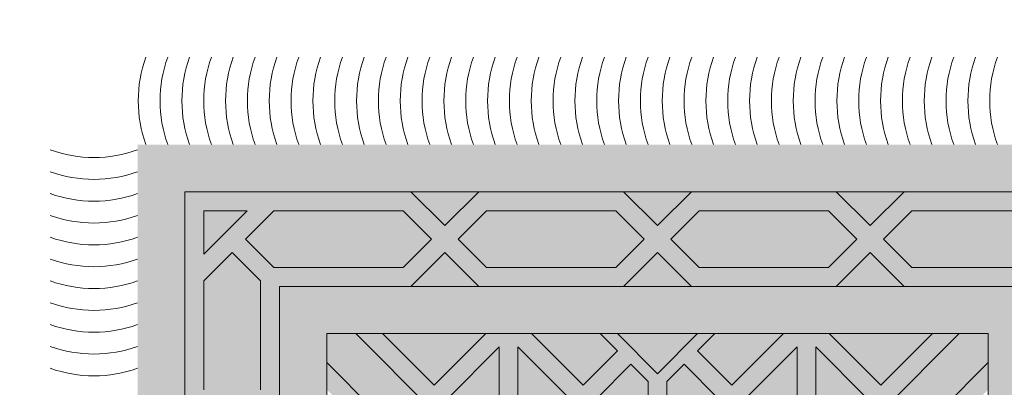
# Model space of a CAD drawing. Units: inches. Extents: x 844 to 2234, y 346 to 1084.
# Tile 21 of 93: x 1114.25 to 1127.54, y 705.06 to 710.02. Entities that reach past the tile are written whole.
import ezdxf

# ---------------------------------------------------------------- set-up
doc = ezdxf.new("R2010")
doc.units = ezdxf.units.IN
doc.header["$MEASUREMENT"] = 0
for name, color, linetype, lineweight in [('A-ANNO-DIMS', 2, 'Continuous', 18), ('furniture', 8, 'Continuous', 18), ('RA-AP-01$0$INT', 35, 'Continuous', 5)]:
    doc.layers.add(name, color=color, linetype=linetype, lineweight=lineweight)
doc.layers.add('RA-AP-01$0$FURN', color=3, linetype='Continuous')
doc.styles.get("Standard").update_dxf_attribs({"font": 'arial.ttf'})
doc.dimstyles.get("Standard").update_dxf_attribs({"dimtxt": 6, "dimasz": 3, "dimexe": 0.18, "dimexo": 0.0625, "dimgap": 0.09, "dimtad": 0, "dimtih": 1, "dimtoh": 1, "dimdec": 1, "dimzin": 0, "dimdsep": 46, "dimlunit": 3, "dimtxsty": 'Standard', "dimblk": 'ARCHTICK', "dimcen": 0.09, "dimadec": 0, "dimazin": 0, "dimtfac": 1, "dimtdec": 1, "dimtofl": 0, "dimtmove": 0, "dimatfit": 3, "dimfxl": 1, "dimtolj": 1, "dimtzin": 0, "dimarcsym": 0})

# ---------------------------------------------------------------- blocks, each defined once
blk = doc.blocks.new('A$C18D01794')
at = {"layer": 'RA-AP-01$0$INT'}
h = blk.add_hatch(color=256, dxfattribs=at)
h.paths.add_polyline_path([(4.3552, -6.1567), (4.3552, -8.0567), (5.4552, -8.0567), (5.4552, -6.1567)])
h.paths.add_polyline_path([(4.4052, -8.0067), (4.4052, -6.2067), (5.4052, -6.2067), (5.4052, -8.0067)], flags=16)
h = blk.add_hatch(color=256, dxfattribs=at)
h.paths.add_polyline_path([(4.5052, -7.5855), (4.4693, -7.5496), (4.5052, -7.5138), (4.5052, -7.382), (4.4693, -7.3461), (4.5052, -7.3102), (4.5052, -7.1784), (4.4693, -7.1426), (4.5052, -7.1067), (4.4769, -7.1067), (4.4552, -7.1284), (4.4335, -7.1067), (4.4052, -7.1067), (4.4411, -7.1426), (4.4052, -7.1784), (4.4052, -7.3102), (4.4411, -7.3461), (4.4052, -7.382), (4.4052, -7.5138), (4.4411, -7.5496), (4.4052, -7.5855), (4.4052, -7.7173), (4.4411, -7.7532), (4.4052, -7.789), (4.4052, -8.0067), (4.6443, -8.0067), (4.6802, -7.9709), (4.7161, -8.0067), (4.8693, -8.0067), (4.9052, -7.9709), (4.9411, -8.0067), (5.0943, -8.0067), (5.1302, -7.9709), (5.1661, -8.0067), (5.4052, -8.0067), (5.4052, -7.789), (5.3693, -7.7532), (5.4052, -7.7173), (5.4052, -7.5855), (5.3693, -7.5496), (5.4052, -7.5138), (5.4052, -7.382), (5.3693, -7.3461), (5.4052, -7.3102), (5.4052, -7.1784), (5.3693, -7.1426), (5.4052, -7.1067), (5.3769, -7.1067), (5.3552, -7.1284), (5.3335, -7.1067), (5.3052, -7.1067), (5.3411, -7.1426), (5.3052, -7.1784), (5.3052, -7.3102), (5.3411, -7.3461), (5.3052, -7.382), (5.3052, -7.5138), (5.3411, -7.5496), (5.3052, -7.5855), (5.3052, -7.7173), (5.3411, -7.7532), (5.3052, -7.789), (5.3052, -7.9067), (5.1661, -7.9067), (5.1302, -7.9426), (5.0943, -7.9067), (4.9411, -7.9067), (4.9052, -7.9426), (4.8693, -7.9067), (4.7161, -7.9067), (4.6802, -7.9426), (4.6443, -7.9067), (4.5052, -7.9067), (4.5052, -7.789), (4.4693, -7.7532), (4.5052, -7.7173)])
h.paths.add_polyline_path([(4.4852, -7.709), (4.4552, -7.739), (4.4252, -7.709), (4.4252, -7.5938), (4.4552, -7.5638), (4.4852, -7.5938)], flags=16)
h.paths.add_polyline_path([(4.4552, -7.7673), (4.4852, -7.7973), (4.4852, -7.9126), (4.4552, -7.9426), (4.4252, -7.9126), (4.4252, -7.7973)], flags=16)
h.paths.add_polyline_path([(4.4552, -7.5355), (4.4252, -7.5055), (4.4252, -7.3902), (4.4552, -7.3602), (4.4852, -7.3902), (4.4852, -7.5055)], flags=16)
h.paths.add_polyline_path([(4.4993, -7.9267), (4.6361, -7.9267), (4.6661, -7.9567), (4.6361, -7.9867), (4.4993, -7.9867), (4.4693, -7.9567)], flags=16)
h.paths.add_polyline_path([(4.4252, -7.9409), (4.4711, -7.9867), (4.4252, -7.9867)], flags=16)
h.paths.add_polyline_path([(4.4552, -7.332), (4.4252, -7.302), (4.4252, -7.1867), (4.4552, -7.1567), (4.4852, -7.1867), (4.4852, -7.302)], flags=16)
h.paths.add_polyline_path([(4.7243, -7.9267), (4.8611, -7.9267), (4.8911, -7.9567), (4.8611, -7.9867), (4.7243, -7.9867), (4.6943, -7.9567)], flags=16)
h.paths.add_polyline_path([(4.9193, -7.9567), (4.9493, -7.9267), (5.0861, -7.9267), (5.1161, -7.9567), (5.0861, -7.9867), (4.9493, -7.9867)], flags=16)
h.paths.add_polyline_path([(5.1443, -7.9567), (5.1743, -7.9267), (5.3111, -7.9267), (5.3411, -7.9567), (5.3111, -7.9867), (5.1743, -7.9867)], flags=16)
h.paths.add_polyline_path([(5.3252, -7.5938), (5.3552, -7.5638), (5.3852, -7.5938), (5.3852, -7.709), (5.3552, -7.739), (5.3252, -7.709)], flags=16)
h.paths.add_polyline_path([(5.3252, -7.7973), (5.3552, -7.7673), (5.3852, -7.7973), (5.3852, -7.9126), (5.3552, -7.9426), (5.3252, -7.9126)], flags=16)
h.paths.add_polyline_path([(5.3252, -7.5055), (5.3252, -7.3902), (5.3552, -7.3602), (5.3852, -7.3902), (5.3852, -7.5055), (5.3552, -7.5355)], flags=16)
h.paths.add_polyline_path([(5.3252, -7.302), (5.3252, -7.1867), (5.3552, -7.1567), (5.3852, -7.1867), (5.3852, -7.302), (5.3552, -7.332)], flags=16)
h.paths.add_polyline_path([(5.3393, -7.9867), (5.3852, -7.9409), (5.3852, -7.9867)], flags=16)
h = blk.add_hatch(color=256, dxfattribs=at)
h.paths.add_polyline_path([(4.4693, -7.1426), (4.5052, -7.1784), (4.5052, -7.1067)])
h.paths.add_polyline_path([(4.4552, -7.1284), (4.4769, -7.1067), (4.4335, -7.1067)])
h.paths.add_polyline_path([(4.4052, -7.1784), (4.4411, -7.1426), (4.4052, -7.1067)])
h.paths.add_polyline_path([(4.4252, -7.302), (4.4552, -7.332), (4.4852, -7.302), (4.4852, -7.1867), (4.4552, -7.1567), (4.4252, -7.1867)])
h.paths.add_polyline_path([(4.5052, -7.382), (4.5052, -7.3102), (4.4693, -7.3461)])
h.paths.add_polyline_path([(4.4252, -7.5055), (4.4552, -7.5355), (4.4852, -7.5055), (4.4852, -7.3902), (4.4552, -7.3602), (4.4252, -7.3902)])
h.paths.add_polyline_path([(4.4252, -7.709), (4.4552, -7.739), (4.4852, -7.709), (4.4852, -7.5938), (4.4552, -7.5638), (4.4252, -7.5938)])
h.paths.add_polyline_path([(4.4693, -7.5496), (4.5052, -7.5855), (4.5052, -7.5138)])
h.paths.add_polyline_path([(4.4052, -7.5855), (4.4411, -7.5496), (4.4052, -7.5138)])
h.paths.add_polyline_path([(4.4052, -7.789), (4.4411, -7.7532), (4.4052, -7.7173)])
h.paths.add_polyline_path([(4.4693, -7.7532), (4.5052, -7.789), (4.5052, -7.7173)])
h.paths.add_polyline_path([(4.4252, -7.9126), (4.4552, -7.9426), (4.4852, -7.9126), (4.4852, -7.7973), (4.4552, -7.7673), (4.4252, -7.7973)])
h.paths.add_polyline_path([(4.4252, -7.9867), (4.4711, -7.9867), (4.4252, -7.9409)])
h.paths.add_polyline_path([(4.4993, -7.9867), (4.6361, -7.9867), (4.6661, -7.9567), (4.6361, -7.9267), (4.4993, -7.9267), (4.4693, -7.9567)])
h.paths.add_polyline_path([(4.6802, -7.9426), (4.7161, -7.9067), (4.6443, -7.9067)])
h.paths.add_polyline_path([(4.6443, -8.0067), (4.7161, -8.0067), (4.6802, -7.9709)])
h.paths.add_polyline_path([(4.7243, -7.9867), (4.8611, -7.9867), (4.8911, -7.9567), (4.8611, -7.9267), (4.7243, -7.9267), (4.6943, -7.9567)])
h.paths.add_polyline_path([(4.9052, -7.9426), (4.9411, -7.9067), (4.8693, -7.9067)])
h.paths.add_polyline_path([(4.8693, -8.0067), (4.9411, -8.0067), (4.9052, -7.9709)])
h.paths.add_polyline_path([(4.9493, -7.9867), (5.0861, -7.9867), (5.1161, -7.9567), (5.0861, -7.9267), (4.9493, -7.9267), (4.9193, -7.9567)])
h.paths.add_polyline_path([(5.1302, -7.9426), (5.1661, -7.9067), (5.0943, -7.9067)])
h.paths.add_polyline_path([(5.0943, -8.0067), (5.1661, -8.0067), (5.1302, -7.9709)])
h.paths.add_polyline_path([(5.1743, -7.9867), (5.3111, -7.9867), (5.3411, -7.9567), (5.3111, -7.9267), (5.1743, -7.9267), (5.1443, -7.9567)])
h.paths.add_polyline_path([(5.3252, -7.9126), (5.3552, -7.9426), (5.3852, -7.9126), (5.3852, -7.7973), (5.3552, -7.7673), (5.3252, -7.7973)])
h.paths.add_polyline_path([(5.3393, -7.9867), (5.3852, -7.9867), (5.3852, -7.9409)])
h.paths.add_polyline_path([(5.3252, -7.709), (5.3552, -7.739), (5.3852, -7.709), (5.3852, -7.5938), (5.3552, -7.5638), (5.3252, -7.5938)])
h.paths.add_polyline_path([(5.3052, -7.789), (5.3411, -7.7532), (5.3052, -7.7173)])
h.paths.add_polyline_path([(5.3693, -7.7532), (5.4052, -7.789), (5.4052, -7.7173)])
h.paths.add_polyline_path([(5.4052, -7.5855), (5.4052, -7.5138), (5.3693, -7.5496)])
h.paths.add_polyline_path([(5.3052, -7.5855), (5.3411, -7.5496), (5.3052, -7.5138)])
h.paths.add_polyline_path([(5.3252, -7.5055), (5.3552, -7.5355), (5.3852, -7.5055), (5.3852, -7.3902), (5.3552, -7.3602), (5.3252, -7.3902)])
h.paths.add_polyline_path([(5.3052, -7.382), (5.3411, -7.3461), (5.3052, -7.3102)])
h.paths.add_polyline_path([(5.3252, -7.302), (5.3552, -7.332), (5.3852, -7.302), (5.3852, -7.1867), (5.3552, -7.1567), (5.3252, -7.1867)])
h.paths.add_polyline_path([(5.4046, -7.3813, -0.001218), (5.4052, -7.3811), (5.4052, -7.3102), (5.3693, -7.3461)])
h.paths.add_polyline_path([(5.3693, -7.1426), (5.4052, -7.1784), (5.4052, -7.1067)])
h.paths.add_polyline_path([(5.3552, -7.1284), (5.3769, -7.1067), (5.3335, -7.1067)])
h.paths.add_polyline_path([(5.3052, -7.1784), (5.3411, -7.1426), (5.3052, -7.1067)])
blk.add_hatch(color=256, dxfattribs=at).paths.add_polyline_path([(4.5052, -7.9067), (5.3052, -7.9067), (5.3052, -7.1067), (5.2552, -7.1067), (5.2552, -7.8567), (4.5552, -7.8567), (4.5552, -7.1067), (4.5052, -7.1067)])
h = blk.add_hatch(color=256, dxfattribs=at)
h.paths.add_polyline_path([(4.5859, -7.8567), (4.6142, -7.8567), (4.6688, -7.8021), (4.7235, -7.8567), (4.7718, -7.8567), (4.8264, -7.8021), (4.8628, -7.8384), (4.8445, -7.8567), (4.8628, -7.8567), (4.9052, -7.8143), (4.9476, -7.8567), (4.9659, -7.8567), (4.9476, -7.8384), (4.984, -7.8021), (5.0386, -7.8567), (5.0869, -7.8567), (5.1416, -7.8021), (5.1962, -7.8567), (5.2245, -7.8567), (4.9052, -7.5374)])
h.paths.add_polyline_path([(4.8952, -7.5757), (4.8952, -7.685), (4.8406, -7.6304)], flags=16)
h.paths.add_polyline_path([(4.9152, -7.5757), (4.9699, -7.6304), (4.9152, -7.685)], flags=16)
h.paths.add_polyline_path([(4.8264, -7.6445), (4.8811, -7.6991), (4.7718, -7.6991)], flags=16)
h.paths.add_polyline_path([(4.984, -7.6445), (5.0386, -7.6991), (4.9293, -7.6991)], flags=16)
h.paths.add_polyline_path([(4.8811, -7.7191), (4.8264, -7.7738), (4.7718, -7.7191)], flags=16)
h.paths.add_polyline_path([(4.9293, -7.7191), (5.0386, -7.7191), (4.984, -7.7738)], flags=16)
h.paths.add_polyline_path([(4.8952, -7.7333), (4.8952, -7.806), (4.8769, -7.8243), (4.8406, -7.7879)], flags=16)
h.paths.add_polyline_path([(4.9152, -7.7333), (4.9699, -7.7879), (4.9335, -7.8243), (4.9152, -7.806)], flags=16)
h.paths.add_polyline_path([(4.7576, -7.7333), (4.8123, -7.7879), (4.7576, -7.8426)], flags=16)
h.paths.add_polyline_path([(4.7376, -7.7333), (4.7376, -7.8426), (4.683, -7.7879)], flags=16)
h.paths.add_polyline_path([(5.0528, -7.7333), (5.0528, -7.8426), (4.9981, -7.7879)], flags=16)
h.paths.add_polyline_path([(5.0728, -7.7333), (5.1274, -7.7879), (5.0728, -7.8426)], flags=16)
h.paths.add_polyline_path([(4.9359, -7.5067), (5.2552, -7.826), (5.2552, -7.7977), (5.2006, -7.7431), (5.2552, -7.6884), (5.2552, -7.6401), (5.2006, -7.5855), (5.2369, -7.5491), (5.2552, -7.5674), (5.2552, -7.5491), (5.2128, -7.5067), (5.2552, -7.4643), (5.2552, -7.446), (5.2369, -7.4643), (5.2006, -7.4279), (5.2552, -7.3733), (5.2552, -7.325), (5.2006, -7.2704), (5.2552, -7.2157), (5.2552, -7.1874)])
h.paths.add_polyline_path([(5.043, -7.4279), (5.0976, -7.3733), (5.0976, -7.4826)], flags=16)
h.paths.add_polyline_path([(5.0288, -7.4421), (5.0835, -7.4967), (4.9742, -7.4967)], flags=16)
h.paths.add_polyline_path([(5.1176, -7.3733), (5.1723, -7.4279), (5.1176, -7.4826)], flags=16)
h.paths.add_polyline_path([(5.0835, -7.5167), (5.0288, -7.5714), (4.9742, -7.5167)], flags=16)
h.paths.add_polyline_path([(5.1318, -7.3591), (5.1864, -7.4138), (5.2411, -7.3591)], flags=17)
h.paths.add_polyline_path([(5.1318, -7.4967), (5.1864, -7.4421), (5.2228, -7.4784), (5.2045, -7.4967)], flags=16)
h.paths.add_polyline_path([(5.0976, -7.5309), (5.0976, -7.6401), (5.043, -7.5855)], flags=16)
h.paths.add_polyline_path([(5.1318, -7.3391), (5.2411, -7.3391), (5.1864, -7.2845)], flags=17)
h.paths.add_polyline_path([(5.1318, -7.5167), (5.2045, -7.5167), (5.2228, -7.535), (5.1864, -7.5714)], flags=16)
h.paths.add_polyline_path([(5.1176, -7.5309), (5.1723, -7.5855), (5.1176, -7.6401)], flags=16)
h.paths.add_polyline_path([(5.1864, -7.5996), (5.2411, -7.6543), (5.1318, -7.6543)], flags=16)
h.paths.add_polyline_path([(5.1318, -7.6743), (5.2411, -7.6743), (5.1864, -7.7289)], flags=16)
h.paths.add_polyline_path([(5.2552, -7.126), (5.2552, -7.1067), (4.5552, -7.1067), (4.5552, -7.126), (4.9052, -7.476)])
h.paths.add_polyline_path([(4.984, -7.3689), (4.9293, -7.3143), (5.0386, -7.3143)], flags=16)
h.paths.add_polyline_path([(4.9699, -7.3831), (4.9152, -7.4377), (4.9152, -7.3284)], flags=16)
h.paths.add_polyline_path([(4.9293, -7.2943), (4.984, -7.2396), (5.0386, -7.2943)], flags=16)
h.paths.add_polyline_path([(5.0528, -7.2801), (4.9981, -7.2255), (5.0528, -7.1709)], flags=16)
h.paths.add_polyline_path([(5.0728, -7.2801), (5.0728, -7.1709), (5.1274, -7.2255)], flags=16)
h.paths.add_polyline_path([(4.8952, -7.4377), (4.8406, -7.3831), (4.8952, -7.3284)], flags=16)
h.paths.add_polyline_path([(4.9152, -7.2801), (4.9152, -7.2074), (4.9335, -7.1891), (4.9699, -7.2255)], flags=16)
h.paths.add_polyline_path([(4.8811, -7.3143), (4.8264, -7.3689), (4.7718, -7.3143)], flags=16)
h.paths.add_polyline_path([(4.8952, -7.2801), (4.8406, -7.2255), (4.8769, -7.1891), (4.8952, -7.2074)], flags=16)
h.paths.add_polyline_path([(4.984, -7.2114), (4.9476, -7.175), (4.9659, -7.1567), (5.0386, -7.1567)], flags=16)
h.paths.add_polyline_path([(4.8811, -7.2943), (4.7718, -7.2943), (4.8264, -7.2396)], flags=16)
h.paths.add_polyline_path([(4.9052, -7.1991), (4.8628, -7.1567), (4.9476, -7.1567)], flags=16)
h.paths.add_polyline_path([(5.1416, -7.2114), (5.0869, -7.1567), (5.1962, -7.1567)], flags=16)
h.paths.add_polyline_path([(4.8264, -7.2114), (4.7718, -7.1567), (4.8445, -7.1567), (4.8628, -7.175)], flags=16)
h.paths.add_polyline_path([(4.8123, -7.2255), (4.7576, -7.2801), (4.7576, -7.1709)], flags=16)
h.paths.add_polyline_path([(4.7376, -7.2801), (4.683, -7.2255), (4.7376, -7.1709)], flags=16)
h.paths.add_polyline_path([(4.7235, -7.1567), (4.6688, -7.2114), (4.6142, -7.1567)], flags=16)
h.paths.add_polyline_path([(4.5976, -7.5067), (4.5552, -7.5491), (4.5552, -7.5674), (4.5735, -7.5491), (4.6099, -7.5855), (4.5552, -7.6401), (4.5552, -7.6884), (4.6099, -7.7431), (4.5552, -7.7977), (4.5552, -7.826), (4.8745, -7.5067), (4.5552, -7.1874), (4.5552, -7.2157), (4.6099, -7.2704), (4.5552, -7.325), (4.5552, -7.3733), (4.6099, -7.4279), (4.5735, -7.4643), (4.5552, -7.446), (4.5552, -7.4643)])
h.paths.add_polyline_path([(4.7128, -7.4826), (4.7128, -7.3733), (4.7674, -7.4279)], flags=16)
h.paths.add_polyline_path([(4.7269, -7.4967), (4.7816, -7.4421), (4.8362, -7.4967)], flags=16)
h.paths.add_polyline_path([(4.6928, -7.4826), (4.6381, -7.4279), (4.6928, -7.3733)], flags=16)
h.paths.add_polyline_path([(4.7269, -7.5167), (4.8362, -7.5167), (4.7816, -7.5714)], flags=16)
h.paths.add_polyline_path([(4.6786, -7.4967), (4.6059, -7.4967), (4.5876, -7.4784), (4.624, -7.4421)], flags=16)
h.paths.add_polyline_path([(4.7128, -7.5309), (4.7674, -7.5855), (4.7128, -7.6401)], flags=16)
h.paths.add_polyline_path([(4.6786, -7.5167), (4.624, -7.5714), (4.5876, -7.535), (4.6059, -7.5167)], flags=16)
h.paths.add_polyline_path([(4.6928, -7.5309), (4.6928, -7.6401), (4.6381, -7.5855)], flags=16)
h.paths.add_polyline_path([(4.624, -7.4138), (4.6786, -7.3591), (4.5693, -7.3591)], flags=17)
h.paths.add_polyline_path([(4.624, -7.5996), (4.6786, -7.6543), (4.5693, -7.6543)], flags=16)
h.paths.add_polyline_path([(4.6786, -7.3391), (4.624, -7.2845), (4.5693, -7.3391)], flags=17)
h.paths.add_polyline_path([(4.6786, -7.6743), (4.624, -7.7289), (4.5693, -7.6743)], flags=16)
h = blk.add_hatch(color=256, dxfattribs=at)
h.paths.add_polyline_path([(4.9052, -7.5374), (4.8745, -7.5067), (4.5552, -7.826), (4.5552, -7.8567), (4.5859, -7.8567)])
h.paths.add_polyline_path([(4.9359, -7.5067), (4.9052, -7.5374), (5.2245, -7.8567), (5.2552, -7.8567), (5.2552, -7.826)])
h.paths.add_polyline_path([(5.2552, -7.1874), (5.2552, -7.126), (4.9052, -7.476), (4.9359, -7.5067)])
h.paths.add_polyline_path([(4.8745, -7.5067), (4.9052, -7.476), (4.5552, -7.126), (4.5552, -7.1874)])
h = blk.add_hatch(color=256, dxfattribs=at)
h.paths.add_polyline_path([(4.9699, -7.6304), (4.9152, -7.5757), (4.9152, -7.685)])
h.paths.add_polyline_path([(4.8952, -7.5757), (4.8406, -7.6304), (4.8952, -7.685)])
h.paths.add_polyline_path([(4.8264, -7.6445), (4.7718, -7.6991), (4.8811, -7.6991)])
h.paths.add_polyline_path([(4.8811, -7.7191), (4.7718, -7.7191), (4.8264, -7.7738)])
h.paths.add_polyline_path([(4.8952, -7.7333), (4.8406, -7.7879), (4.8769, -7.8243), (4.8952, -7.806)])
h.paths.add_polyline_path([(4.8628, -7.8384), (4.8264, -7.8021), (4.7718, -7.8567), (4.8445, -7.8567)])
h.paths.add_polyline_path([(4.8123, -7.7879), (4.7576, -7.7333), (4.7576, -7.8426)])
h.paths.add_polyline_path([(4.7376, -7.7333), (4.683, -7.7879), (4.7376, -7.8426)])
h.paths.add_polyline_path([(4.6688, -7.8021), (4.6142, -7.8567), (4.7235, -7.8567)])
h.paths.add_polyline_path([(4.9052, -7.8143), (4.8628, -7.8567), (4.9476, -7.8567)])
h.paths.add_polyline_path([(4.9152, -7.7333), (4.9152, -7.806), (4.9335, -7.8243), (4.9699, -7.7879)])
h.paths.add_polyline_path([(5.0386, -7.7191), (4.9293, -7.7191), (4.984, -7.7738)])
h.paths.add_polyline_path([(4.984, -7.6445), (4.9293, -7.6991), (5.0386, -7.6991)])
h.paths.add_polyline_path([(5.0528, -7.7333), (4.9981, -7.7879), (5.0528, -7.8426)])
h.paths.add_polyline_path([(4.984, -7.8021), (4.9476, -7.8384), (4.9659, -7.8567), (5.0386, -7.8567)])
h.paths.add_polyline_path([(5.1274, -7.7879), (5.0728, -7.7333), (5.0728, -7.8426)])
h.paths.add_polyline_path([(5.1416, -7.8021), (5.0869, -7.8567), (5.1962, -7.8567)])
for p, q in [((4.5552, -7.1067), (4.5552, -7.8567)), ((5.2552, -7.1067), (5.2552, -7.8567)), ((4.8745, -7.5067), (4.5552, -7.826)), ((4.9359, -7.5067), (5.2552, -7.826)), ((4.9052, -7.5374), (4.5859, -7.8567)), ((4.9052, -7.5374), (5.2245, -7.8567)), ((4.7376, -7.7333), (4.7376, -7.8426)), ((4.7576, -7.7333), (4.7576, -7.8426)), ((4.8952, -7.806), (4.8952, -7.7333)), ((4.9152, -7.806), (4.9152, -7.7333)), ((5.0528, -7.7333), (5.0528, -7.8426)), ((5.0728, -7.7333), (5.0728, -7.8426)), ((4.7376, -7.8426), (4.683, -7.7879)), ((4.7576, -7.8426), (4.8123, -7.7879)), ((4.8406, -7.7879), (4.8769, -7.8243)), ((4.9699, -7.7879), (4.9335, -7.8243)), ((5.0528, -7.8426), (4.9981, -7.7879)), ((5.0728, -7.8426), (5.1274, -7.7879)), ((4.4252, -7.7973), (4.4252, -7.9126)), ((4.4852, -7.9126), (4.4852, -7.7973)), ((4.6142, -7.8567), (4.6688, -7.8021)), ((4.7235, -7.8567), (4.6688, -7.8021)), ((4.7718, -7.8567), (4.8264, -7.8021)), ((4.8264, -7.8021), (4.8628, -7.8384)), ((4.984, -7.8021), (4.9476, -7.8384)), ((5.0386, -7.8567), (4.984, -7.8021)), ((5.0869, -7.8567), (5.1416, -7.8021)), ((5.1962, -7.8567), (5.1416, -7.8021)), ((4.8952, -7.806), (4.8769, -7.8243)), ((4.9152, -7.806), (4.9335, -7.8243)), ((4.9052, -7.8143), (4.8628, -7.8567)), ((4.9052, -7.8143), (4.9476, -7.8567)), ((4.8445, -7.8567), (4.8628, -7.8384)), ((4.9476, -7.8384), (4.9659, -7.8567)), ((4.9659, -7.8567), (4.9476, -7.8384)), ((4.5552, -7.8567), (5.2552, -7.8567)), ((4.8445, -7.8567), (4.7718, -7.8567)), ((4.9476, -7.8567), (4.8628, -7.8567)), ((4.9659, -7.8567), (5.0386, -7.8567)), ((4.4252, -7.9126), (4.4552, -7.9426)), ((4.4852, -7.9126), (4.4552, -7.9426)), ((5.2672, -7.9067), (4.5432, -7.9067)), ((5.2672, -7.9067), (4.5432, -7.9067)), ((4.6443, -7.9067), (4.6802, -7.9426)), ((4.7161, -7.9067), (4.6802, -7.9426)), ((4.8693, -7.9067), (4.9052, -7.9426)), ((4.9411, -7.9067), (4.9052, -7.9426)), ((5.0943, -7.9067), (5.1302, -7.9426)), ((5.1661, -7.9067), (5.1302, -7.9426)), ((4.4993, -7.9267), (4.4693, -7.9567)), ((4.6361, -7.9267), (4.4993, -7.9267)), ((4.6361, -7.9267), (4.6661, -7.9567)), ((4.7243, -7.9267), (4.6943, -7.9567)), ((4.8611, -7.9267), (4.7243, -7.9267)), ((4.8611, -7.9267), (4.8911, -7.9567)), ((4.9493, -7.9267), (4.9193, -7.9567)), ((4.9493, -7.9267), (5.0861, -7.9267)), ((5.0861, -7.9267), (5.1161, -7.9567)), ((5.1743, -7.9267), (5.1443, -7.9567)), ((5.1743, -7.9267), (5.3111, -7.9267)), ((4.4252, -7.9409), (4.4252, -7.9867)), ((4.4711, -7.9867), (4.4252, -7.9409)), ((4.4993, -7.9867), (4.4693, -7.9567)), ((4.6361, -7.9867), (4.6661, -7.9567)), ((4.7243, -7.9867), (4.6943, -7.9567)), ((4.8611, -7.9867), (4.8911, -7.9567)), ((4.9493, -7.9867), (4.9193, -7.9567)), ((5.0861, -7.9867), (5.1161, -7.9567)), ((5.1743, -7.9867), (5.1443, -7.9567)), ((4.6443, -8.0067), (4.6802, -7.9709)), ((4.7161, -8.0067), (4.6802, -7.9709)), ((4.8693, -8.0067), (4.9052, -7.9709)), ((4.9411, -8.0067), (4.9052, -7.9709)), ((5.0943, -8.0067), (5.1302, -7.9709)), ((5.1661, -8.0067), (5.1302, -7.9709)), ((4.4711, -7.9867), (4.4252, -7.9867)), ((4.6361, -7.9867), (4.4993, -7.9867)), ((4.8611, -7.9867), (4.7243, -7.9867)), ((4.9493, -7.9867), (5.0861, -7.9867)), ((5.1743, -7.9867), (5.3111, -7.9867))]:
    blk.add_line(p, q, dxfattribs=at)
for points in [[(5.4052, -8.0067), (4.4052, -8.0067), (4.4052, -7.1067)], [(5.3052, -7.1067), (5.3052, -7.9067), (4.5052, -7.9067), (4.5052, -7.1067)]]:
    blk.add_lwpolyline(points, dxfattribs=at)
for centre, start, end in [((4.309, -7.9484), 70.2038, 109.7962), ((4.309, -7.9715), 70.2038, 109.7962), ((4.309, -7.9946), 70.2038, 109.7962), ((4.309, -8.0177), 70.2038, 109.7962), ((4.309, -8.0408), 70.2038, 109.7962), ((4.309, -8.0639), 70.2038, 109.7962), ((4.309, -8.087), 70.2038, 109.7962), ((4.309, -8.1101), 70.2038, 109.7962), ((4.309, -8.1332), 70.2038, 109.7962), ((4.309, -8.1563), 70.2038, 109.7962), ((4.309, -8.1794), 70.2038, 109.7962), ((4.4922, -8.1029), 160.2038, 199.7962), ((4.5153, -8.1029), 160.2038, 199.7962), ((4.5384, -8.1029), 160.2038, 199.7962), ((4.5615, -8.1029), 160.2038, 199.7962), ((4.5846, -8.1029), 160.2038, 199.7962), ((4.6077, -8.1029), 160.2038, 199.7962), ((4.6308, -8.1029), 160.2038, 199.7962), ((4.6539, -8.1029), 160.2038, 199.7962), ((4.677, -8.1029), 160.2038, 199.7962), ((4.7001, -8.1029), 160.2038, 199.7962), ((4.7232, -8.1029), 160.2038, 199.7962), ((4.7463, -8.1029), 160.2038, 199.7962), ((4.7694, -8.1029), 160.2038, 199.7962), ((4.7925, -8.1029), 160.2038, 199.7962), ((4.8156, -8.1029), 160.2038, 199.7962), ((4.8387, -8.1029), 160.2038, 199.7962), ((4.8618, -8.1029), 160.2038, 199.7962), ((4.8849, -8.1029), 160.2038, 199.7962), ((4.908, -8.1029), 160.2038, 199.7962), ((4.9311, -8.1029), 160.2038, 199.7962), ((4.9542, -8.1029), 160.2038, 199.7962), ((4.9773, -8.1029), 160.2038, 199.7962), ((5.0004, -8.1029), 160.2038, 199.7962), ((5.0235, -8.1029), 160.2038, 199.7962), ((5.0466, -8.1029), 160.2038, 199.7962), ((5.0697, -8.1029), 160.2038, 199.7962), ((5.0928, -8.1029), 160.2038, 199.7962), ((5.1159, -8.1029), 160.2038, 199.7962), ((5.139, -8.1029), 160.2038, 199.7962), ((5.1621, -8.1029), 160.2038, 199.7962), ((5.1852, -8.1029), 160.2038, 199.7962), ((5.2083, -8.1029), 160.2038, 199.7962), ((5.2314, -8.1029), 160.2038, 199.7962), ((5.2545, -8.1029), 160.2038, 199.7962), ((5.2776, -8.1029), 160.2038, 199.7962), ((5.3007, -8.1029), 160.2038, 199.7962), ((5.3238, -8.1029), 160.2038, 199.7962), ((5.3469, -8.1029), 160.2038, 199.7962), ((5.37, -8.1029), 160.2038, 199.7962), ((5.3931, -8.1029), 160.2038, 199.7962)]:
    blk.add_arc(centre, 0.1364, start, end, dxfattribs=at)
blk = doc.blocks.new('A$C5D2F253E')
at = {"layer": 'RA-AP-01$0$FURN', "xscale": -0.7999999999883585, "yscale": 0.7999999999883585, "zscale": 0.8, "rotation": 90}
blk.add_blockref('A$C18D01794', (-5.68776, 4.75792), dxfattribs=at)
blk = doc.blocks.new('_ArchTick')
at = {"color": 0, "linetype": 'ByBlock', "const_width": 0.15}
blk.add_lwpolyline([(-0.5, -0.5), (0.5, 0.5)], dxfattribs=at)
blk = doc.blocks.new('*D144')
at = {"layer": 'A-ANNO-DIMS', "color": 0, "lineweight": -2, "transparency": 16777216}
for p, q in [((1096.616, 439.373), (1096.616, 1074.743)), ((1143.116, 492.373), (1143.116, 1074.743)), ((1096.616, 1074.563), (1102.482, 1074.563)), ((1143.116, 1074.563), (1137.25, 1074.563))]:
    blk.add_line(p, q, dxfattribs=at)
at = {"layer": 'Defpoints', "color": 0, "transparency": 16777216}
for p in [(1143.116, 1074.563), (1143.116, 492.311), (1096.616, 439.311)]:
    blk.add_point(p, dxfattribs=at)
at = {"layer": 'A-ANNO-DIMS', "color": 0, "lineweight": -2, "transparency": 16777216, "xscale": 3, "yscale": 3, "zscale": 3, "rotation": 180}
blk.add_blockref('_ArchTick', (1096.616, 1074.563), dxfattribs=at)
at = {"layer": 'A-ANNO-DIMS', "color": 0, "lineweight": -2, "transparency": 16777216, "xscale": 3, "yscale": 3, "zscale": 3}
blk.add_blockref('_ArchTick', (1143.116, 1074.563), dxfattribs=at)
at = {"layer": 'A-ANNO-DIMS', "color": 0, "transparency": 16777216, "insert": (1119.866, 1074.563), "char_height": 6, "attachment_point": 5}
blk.add_mtext('\\A1;3\'-10 1/2"', dxfattribs=at)

msp = doc.modelspace()

# ---------------------------------------------------------------- block references
at = {"layer": 'furniture', "xscale": 15.94108302203742, "yscale": 15.94108302203742, "zscale": 15.94108302203742, "rotation": 90}
msp.add_blockref('A$C5D2F253E', (1136.148, 696.258), dxfattribs=at)

# ---------------------------------------------------------------- dimensions: what is measured, and where the dimension line sits
at = {"layer": 'A-ANNO-DIMS'}
dim = msp.add_linear_dim(base=(1143.116, 1074.563), p1=(1096.616, 439.311), p2=(1143.116, 492.311), dimstyle='Standard', override={"dimdec": 1, "dimlfac": 1, "dimrnd": 0, "dimzin": 1, "dimdsep": 46, "dimlunit": 4, "dimfrac": 2}, dxfattribs=at)
dim.commit()
dim.dimension.update_dxf_attribs({"geometry": '*D144', "text_midpoint": (1119.866, 1074.563)})

doc.saveas('drawing.dxf')
